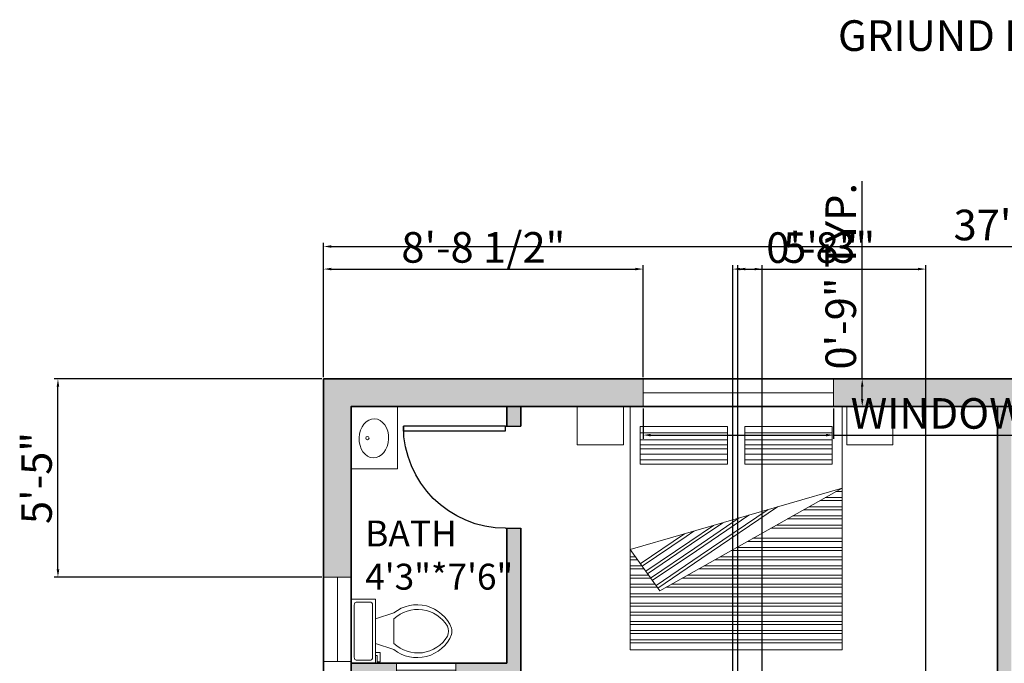
# Model space of a CAD drawing. Units: inches. Extents: x 1698 to 2352, y 1975 to 2732.
# Tile 3 of 4: x 1707 to 2029, y 2521 to 2732. Entities that reach past the tile are written whole.
import ezdxf

# ---------------------------------------------------------------- set-up
doc = ezdxf.new("R2010")
doc.units = ezdxf.units.IN
for name, color, linetype, lineweight in [('A-ANNO-DIMS', 2, 'Continuous', 18), ('A-ANNO-TEXT', 7, 'Continuous', 25), ('A-AREA-IDEN', 7, 'Continuous', 18), ('A-FLOR-FIXT', 231, 'Continuous', 18), ('A-WALL-PATT', 52, 'Continuous', 13), ('door', 80, 'Continuous', 25), ('fur', 10, 'Continuous', 18), ('wall', 7, 'Continuous', 35), ('window', 130, 'Continuous', 18)]:
    doc.layers.add(name, color=color, linetype=linetype, lineweight=lineweight)
doc.styles.get("Standard").update_dxf_attribs({"font": 'arial.ttf'})
doc.dimstyles.new('ISO-25', dxfattribs={"dimtxt": 10, "dimasz": 2.5, "dimexe": 1.25, "dimexo": 0.625, "dimtad": 1, "dimdec": 0, "dimlunit": 4, "dimtxsty": 'Standard', "dimcen": 2.5, "dimadec": 0, "dimazin": 0, "dimtfac": 1, "dimtdec": 0, "dimtmove": 0, "dimatfit": 3, "dimfxl": 1, "dimarcsym": 0})

# ---------------------------------------------------------------- blocks, each defined once
blk = doc.blocks.new('*U2')
for p, q in [((0, 0), (0, -6)), ((40, 0), (40, -6))]:
    blk.add_line(p, q)
blk.add_lwpolyline([(0, 0), (0, 40), (1.75, 40), (1.75, 0)], close=True)
blk.add_arc((0, 0), 40, 0, 90)
blk = doc.blocks.new('*U4')
for p, q in [((9.5, -6), (9.5, -2)), ((-10, -8.5), (-8, -8.5)), ((-10, -9.5), (-10, -8.5)), ((-7, -9.5), (-10, -9.5)), ((-8, -8.5), (-8, -8)), ((-7, -8), (-7, -9.5)), ((-4, -8), (-6, -14)), ((4, -8), (6, -14)), ((4, -14), (-4, -14))]:
    blk.add_line(p, q)
blk.add_lwpolyline([(10.5, -8), (10.5, 0), (-10.5, 0), (-10.5, -8)], close=True)
for points in [[(-9.5, -2), (-9.5, -6)], [(8.5, -1), (-8.5, -1)], [(-8.5, -7), (8.5, -7)]]:
    blk.add_lwpolyline(points)
for centre, radius, start, end in [((-8.62, -1.88), 0.884, 81.8699, 188.1301), ((8.62, -1.88), 0.884, 351.8699, 98.1301), ((-8.62, -6.12), 0.884, 171.8699, 278.1301), ((8.62, -6.12), 0.884, 261.8699, 8.1301), ((3.52, -21.58), 12.17, 141.4691, 247.9714), ((4.2, -21.82), 11.33, 136.3677, 238.9468), ((-3.52, -21.58), 12.17, 292.0284, 38.5307), ((-4.2, -21.82), 11.33, 301.053, 43.6321), ((0, -27.88), 4, 245.7318, 294.2682), ((0, -29), 4, 254.8605, 285.1395)]:
    blk.add_arc(centre, radius, start, end)
blk = doc.blocks.new('*D7')
at = {"layer": 'A-ANNO-DIMS', "color": 0, "lineweight": -2, "transparency": 16777216}
for p, q in [((1805.99, 2614.89), (1805.99, 2658.85)), ((2255.99, 2614.89), (2255.99, 2658.85)), ((1808.49, 2657.6), (2253.49, 2657.6))]:
    blk.add_line(p, q, dxfattribs=at)
at = {"layer": 'A-ANNO-DIMS', "color": 0, "lineweight": 100, "transparency": 16777216}
for points in [[(1808.49, 2658.02), (1808.49, 2657.18), (1805.99, 2657.6)], [(2253.49, 2658.02), (2253.49, 2657.18), (2255.99, 2657.6)]]:
    blk.add_solid(points, dxfattribs=at)
at = {"layer": 'Defpoints', "color": 0, "lineweight": 100, "transparency": 16777216}
for p in [(2255.99, 2657.6), (1805.99, 2614.26), (2255.99, 2614.26)]:
    blk.add_point(p, dxfattribs=at)
at = {"layer": 'A-ANNO-DIMS', "color": 0, "transparency": 16777216, "insert": (2030.99, 2663.33), "char_height": 10, "attachment_point": 5}
blk.add_mtext('37\'-6"', dxfattribs=at)
blk = doc.blocks.new('BED-DOUBLE-WITH-NIGHTSTANDS')
for p, q in [((20.55, 70.98), (49.18, 70.98)), ((54.81, 70.98), (83.45, 70.98)), ((20.61, 68.69), (49.25, 68.69)), ((54.87, 68.69), (83.51, 68.69)), ((20.55, 67.05), (49.18, 67.05)), ((20.55, 65.74), (49.18, 65.74)), ((54.81, 67.05), (83.45, 67.05)), ((54.81, 65.74), (83.45, 65.74)), ((20.55, 63.98), (49.18, 63.98)), ((20.55, 62.15), (49.18, 62.15)), ((54.81, 63.98), (83.45, 63.98)), ((54.81, 62.15), (83.45, 62.15)), ((17.28, 32.76), (86.63, 52.89)), ((86.63, 52.89), (27, 19.28)), ((84.66, 51.78), (86.63, 51.78)), ((86.25, 52.78), (86.63, 52.78)), ((79.34, 48.78), (86.63, 48.78)), ((81.11, 49.78), (86.63, 49.78)), ((40.19, 30.78), (62.43, 45.87)), ((40.75, 29.96), (65.55, 46.77)), ((74.02, 45.78), (86.63, 45.78)), ((75.79, 46.78), (86.63, 46.78)), ((38.42, 33.24), (53.01, 43.13)), ((38.98, 32.41), (56.13, 44.04)), ((68.7, 42.78), (86.63, 42.78)), ((70.47, 43.78), (86.63, 43.78)), ((35.61, 37.09), (38.16, 38.82)), ((36.83, 35.44), (44.53, 40.67)), ((37.39, 34.62), (47.65, 41.57)), ((63.38, 39.78), (86.63, 39.78)), ((65.15, 40.78), (86.63, 40.78)), ((20.62, 28.13), (35.05, 37.91)), ((21.18, 27.3), (35.61, 37.09)), ((55.69, 35.45), (86.63, 35.45)), ((57.46, 36.45), (86.63, 36.45)), ((27, 19.28), (17.28, 32.76)), ((17.28, 32.45), (17.5, 32.45)), ((22.4, 25.66), (36.83, 35.44)), ((22.96, 24.83), (37.39, 34.62)), ((23.99, 23.45), (38.42, 33.24)), ((24.55, 22.62), (38.98, 32.41)), ((50.37, 32.45), (86.63, 32.45)), ((52.14, 33.45), (86.63, 33.45)), ((17.28, 30.45), (18.94, 30.45)), ((17.28, 29.45), (19.66, 29.45)), ((25.76, 21), (40.19, 30.78)), ((26.32, 20.17), (40.75, 29.96)), ((45.05, 29.45), (86.63, 29.45)), ((46.82, 30.45), (86.63, 30.45)), ((17.28, 27.45), (21.11, 27.45)), ((17.28, 26.45), (21.83, 26.45)), ((39.73, 26.45), (86.63, 26.45)), ((41.5, 27.45), (86.63, 27.45)), ((17.28, 24.45), (23.27, 24.45)), ((17.28, 23.45), (23.99, 23.45)), ((34.41, 23.45), (86.63, 23.45)), ((36.18, 24.45), (86.63, 24.45)), ((17.28, 21.45), (25.43, 21.45)), ((17.28, 20.45), (26.16, 20.45)), ((29.09, 20.45), (86.63, 20.45)), ((30.86, 21.45), (86.63, 21.45)), ((17.28, 18.28), (86.63, 18.28)), ((17.28, 17.28), (86.63, 17.28)), ((17.28, 15.28), (86.63, 15.28)), ((17.28, 14.28), (86.63, 14.28)), ((17.28, 12.28), (86.63, 12.28)), ((17.28, 11.28), (86.63, 11.28)), ((17.28, 9.28), (86.63, 9.28)), ((17.28, 8.28), (86.63, 8.28)), ((17.28, 6.28), (86.63, 6.28)), ((17.28, 5.28), (86.63, 5.28)), ((17.28, 3.28), (86.63, 3.28)), ((17.28, 2.28), (86.63, 2.28))]:
    blk.add_line(p, q)
for points in [[(0, 79.57), (15.07, 79.57), (15.07, 67), (0, 67)], [(17.28, 79.57), (86.63, 79.57), (86.63, 0), (17.28, 0)], [(88.18, 79.57), (103.25, 79.57), (103.25, 67), (88.18, 67)], [(20.55, 73), (49.18, 73), (49.18, 60.76), (20.55, 60.76)], [(54.81, 73), (83.45, 73), (83.45, 60.76), (54.81, 60.76)]]:
    blk.add_lwpolyline(points, close=True)
blk = doc.blocks.new('BASIN-VANITY')
blk.add_lwpolyline([(0, 20.39), (15.22, 20.39), (15.22, 0), (0, 0)], close=True)
blk.add_circle((5.32, 10.07), 0.551)
blk.add_ellipse((7.43, 9.98), major_axis=(-0.23, -6.4), ratio=0.75221)
blk = doc.blocks.new('WIN-BATH-19_41')
blk.add_line((0, 2.25), (19.41, 2.25))
blk.add_lwpolyline([(0, 4.5), (19.41, 4.5), (19.41, 0), (0, 0)], close=True)
blk = doc.blocks.new('WIN-BATH-27_578')
blk.add_line((4.5, 0), (4.5, 27.58))
blk.add_lwpolyline([(0, 0), (9, 0), (9, 27.58), (0, 27.58)], close=True)
blk = doc.blocks.new('WIN-BEDROOM-62_374')
blk.add_line((0, 4.5), (62.37, 4.5))
blk.add_lwpolyline([(0, 0), (62.37, 0), (62.37, 9), (0, 9)], close=True)
blk = doc.blocks.new('*D20')
at = {"layer": 'A-ANNO-DIMS', "color": 0, "lineweight": -2, "transparency": 16777216}
for p, q in [((2046.1, 2605.26), (2046.1, 2693.32)), ((2060.97, 2605.26), (2044.85, 2605.26)), ((2046.1, 2528.19), (2046.1, 2602.76)), ((2060.97, 2525.69), (2044.85, 2525.69))]:
    blk.add_line(p, q, dxfattribs=at)
at = {"layer": 'A-ANNO-DIMS', "color": 0, "lineweight": 100, "transparency": 16777216}
for points in [[(2045.69, 2602.76), (2046.52, 2602.76), (2046.1, 2605.26)], [(2045.69, 2528.19), (2046.52, 2528.19), (2046.1, 2525.69)]]:
    blk.add_solid(points, dxfattribs=at)
at = {"layer": 'Defpoints', "color": 0, "lineweight": 100, "transparency": 16777216}
for p in [(2046.1, 2605.26), (2061.59, 2605.26), (2061.59, 2525.69)]:
    blk.add_point(p, dxfattribs=at)
at = {"layer": 'A-ANNO-DIMS', "color": 0, "transparency": 16777216, "insert": (2040.31, 2650.54), "char_height": 10, "attachment_point": 5, "rotation": 90}
blk.add_mtext('6\'-7 1/2" TYP.', dxfattribs=at)
blk = doc.blocks.new('*D29')
at = {"layer": 'A-ANNO-DIMS', "color": 0, "lineweight": -2, "transparency": 16777216}
for p, q in [((1910.52, 2604.64), (1910.52, 2594.66)), ((1972.89, 2604.64), (1972.89, 2594.66)), ((1913.02, 2595.91), (1970.39, 2595.91)), ((1972.89, 2595.91), (2126.48, 2595.91))]:
    blk.add_line(p, q, dxfattribs=at)
at = {"layer": 'A-ANNO-DIMS', "color": 0, "lineweight": 100, "transparency": 16777216}
for points in [[(1913.02, 2596.32), (1913.02, 2595.49), (1910.52, 2595.91)], [(1970.39, 2596.32), (1970.39, 2595.49), (1972.89, 2595.91)]]:
    blk.add_solid(points, dxfattribs=at)
at = {"layer": 'Defpoints', "color": 0, "lineweight": 100, "transparency": 16777216}
for p in [(1910.52, 2605.26), (1972.89, 2605.26), (1972.89, 2595.91)]:
    blk.add_point(p, dxfattribs=at)
at = {"layer": 'A-ANNO-DIMS', "color": 0, "transparency": 16777216, "insert": (2050.94, 2601.7), "char_height": 10, "attachment_point": 5}
blk.add_mtext('WINDOW 5\'-2 1/2" TYP.', dxfattribs=at)
blk = doc.blocks.new('*D30')
at = {"layer": 'A-ANNO-DIMS', "color": 0, "lineweight": -2, "transparency": 16777216}
for p, q in [((1982.25, 2614.26), (1982.25, 2678.97)), ((1973.52, 2614.26), (1983.5, 2614.26)), ((1982.25, 2607.76), (1982.25, 2611.76)), ((1973.52, 2605.26), (1983.5, 2605.26))]:
    blk.add_line(p, q, dxfattribs=at)
at = {"layer": 'A-ANNO-DIMS', "color": 0, "lineweight": 100, "transparency": 16777216}
for points in [[(1981.83, 2611.76), (1982.66, 2611.76), (1982.25, 2614.26)], [(1981.83, 2607.76), (1982.66, 2607.76), (1982.25, 2605.26)]]:
    blk.add_solid(points, dxfattribs=at)
at = {"layer": 'Defpoints', "color": 0, "lineweight": 100, "transparency": 16777216}
for p in [(1972.89, 2614.26), (1982.25, 2614.26), (1972.89, 2605.26)]:
    blk.add_point(p, dxfattribs=at)
at = {"layer": 'A-ANNO-DIMS', "color": 0, "transparency": 16777216, "insert": (1976.52, 2647.86), "char_height": 10, "attachment_point": 5, "rotation": 90}
blk.add_mtext('0\'-9" TYP.', dxfattribs=at)
blk = doc.blocks.new('*D36')
at = {"layer": 'A-ANNO-DIMS', "color": 0, "lineweight": -2, "transparency": 16777216}
for p, q in [((1941.49, 2286.14), (1941.49, 2651.46)), ((1943.99, 2650.21), (1946.99, 2650.21)), ((1949.49, 2286.14), (1949.49, 2651.46)), ((1949.49, 2650.21), (1979.82, 2650.21))]:
    blk.add_line(p, q, dxfattribs=at)
at = {"layer": 'A-ANNO-DIMS', "color": 0, "lineweight": 100, "transparency": 16777216}
for points in [[(1943.99, 2650.63), (1943.99, 2649.8), (1941.49, 2650.21)], [(1946.99, 2650.63), (1946.99, 2649.8), (1949.49, 2650.21)]]:
    blk.add_solid(points, dxfattribs=at)
at = {"layer": 'Defpoints', "color": 0, "lineweight": 100, "transparency": 16777216}
for p in [(1949.49, 2650.21), (1941.49, 2285.51), (1949.49, 2285.51)]:
    blk.add_point(p, dxfattribs=at)
at = {"layer": 'A-ANNO-DIMS', "color": 0, "transparency": 16777216, "insert": (1965.91, 2655.94), "char_height": 10, "attachment_point": 5}
blk.add_mtext('0\'-8"', dxfattribs=at)
blk = doc.blocks.new('*D40')
at = {"layer": 'A-ANNO-DIMS', "color": 0, "lineweight": -2, "transparency": 16777216}
for p, q in [((1805.99, 2614.89), (1805.99, 2651.46)), ((1808.49, 2650.21), (1908.02, 2650.21)), ((1910.52, 2614.89), (1910.52, 2651.46))]:
    blk.add_line(p, q, dxfattribs=at)
at = {"layer": 'A-ANNO-DIMS', "color": 0, "lineweight": 100, "transparency": 16777216}
for points in [[(1808.49, 2650.63), (1808.49, 2649.8), (1805.99, 2650.21)], [(1908.02, 2650.63), (1908.02, 2649.8), (1910.52, 2650.21)]]:
    blk.add_solid(points, dxfattribs=at)
at = {"layer": 'Defpoints', "color": 0, "lineweight": 100, "transparency": 16777216}
for p in [(1910.52, 2650.21), (1805.99, 2614.26), (1910.52, 2614.26)]:
    blk.add_point(p, dxfattribs=at)
at = {"layer": 'A-ANNO-DIMS', "color": 0, "transparency": 16777216, "insert": (1858.25, 2656.01), "char_height": 10, "attachment_point": 5}
blk.add_mtext('8\'-8 1/2"', dxfattribs=at)
blk = doc.blocks.new('*D43')
at = {"layer": 'A-ANNO-DIMS', "color": 0, "lineweight": -2, "transparency": 16777216}
for p, q in [((1805.37, 2614.26), (1717.79, 2614.26)), ((1719.04, 2551.97), (1719.04, 2611.76)), ((1805.37, 2549.47), (1717.79, 2549.47))]:
    blk.add_line(p, q, dxfattribs=at)
at = {"layer": 'A-ANNO-DIMS', "color": 0, "lineweight": 100, "transparency": 16777216}
for points in [[(1718.62, 2611.76), (1719.46, 2611.76), (1719.04, 2614.26)], [(1718.62, 2551.97), (1719.46, 2551.97), (1719.04, 2549.47)]]:
    blk.add_solid(points, dxfattribs=at)
at = {"layer": 'Defpoints', "color": 0, "lineweight": 100, "transparency": 16777216}
for p in [(1719.04, 2614.26), (1805.99, 2614.26), (1805.99, 2549.47)]:
    blk.add_point(p, dxfattribs=at)
at = {"layer": 'A-ANNO-DIMS', "color": 0, "transparency": 16777216, "insert": (1713.33, 2581.87), "char_height": 10, "attachment_point": 5, "rotation": 90}
blk.add_mtext('5\'-5"', dxfattribs=at)
blk = doc.blocks.new('*D50')
at = {"layer": 'A-ANNO-DIMS', "color": 0, "lineweight": -2, "transparency": 16777216}
for p, q in [((1939.87, 2337.39), (1939.87, 2651.46)), ((1942.37, 2650.21), (2000.54, 2650.21)), ((2003.04, 2337.39), (2003.04, 2651.46))]:
    blk.add_line(p, q, dxfattribs=at)
at = {"layer": 'A-ANNO-DIMS', "color": 0, "lineweight": 100, "transparency": 16777216}
for points in [[(1942.37, 2650.63), (1942.37, 2649.8), (1939.87, 2650.21)], [(2000.54, 2650.63), (2000.54, 2649.8), (2003.04, 2650.21)]]:
    blk.add_solid(points, dxfattribs=at)
at = {"layer": 'Defpoints', "color": 0, "lineweight": 100, "transparency": 16777216}
for p in [(2003.04, 2650.21), (1939.87, 2336.76), (2003.04, 2336.76)]:
    blk.add_point(p, dxfattribs=at)
at = {"layer": 'A-ANNO-DIMS', "color": 0, "transparency": 16777216, "insert": (1971.45, 2655.95), "char_height": 10, "attachment_point": 5}
blk.add_mtext('5\'-3"', dxfattribs=at)

msp = doc.modelspace()

# ---------------------------------------------------------------- hatches: boundary and pattern name
at = {"layer": 'A-WALL-PATT'}
h = msp.add_hatch(color=256, dxfattribs=at)
h.dxf.hatch_style = 1
h.paths.add_polyline_path([(1910.52, 2614.26), (1805.99, 2614.26), (1805.99, 2549.47), (1814.99, 2549.47), (1814.99, 2605.26), (1910.52, 2605.26)])
h.paths.add_polyline_path([(2084.19, 2614.26), (1972.89, 2614.26), (1972.89, 2605.26), (2026.49, 2605.26), (2084.19, 2605.26)])
h.paths.add_polyline_path([(2255.99, 2614.26), (2146.56, 2614.26), (2146.56, 2605.26), (2148.21, 2605.26), (2186.99, 2605.26), (2246.99, 2605.26), (2246.99, 2546.53), (2255.99, 2546.53)])
h.paths.add_polyline_path([(2191.49, 2605.26), (2186.99, 2605.26), (2186.99, 2595.02), (2191.49, 2595.02)], flags=17)
h.paths.add_polyline_path([(2191.49, 2563.28), (2186.99, 2563.28), (2186.99, 2510.76), (2191.49, 2510.76)])
h.paths.add_polyline_path([(2246.99, 2515.26), (2191.49, 2515.26), (2191.49, 2510.76), (2246.99, 2510.76)])
h.paths.add_polyline_path([(2030.99, 2605.26), (2026.49, 2605.26), (2026.49, 2473.26), (2020.85, 2473.26), (2020.85, 2468.76), (2030.99, 2468.76)])
h.paths.add_polyline_path([(1980.85, 2473.26), (1870.49, 2473.26), (1865.99, 2473.26), (1865.99, 2468.76), (1980.85, 2468.76)])
h.paths.add_polyline_path([(1828.36, 2413.26), (1814.99, 2413.26), (1814.99, 2408.76), (1828.36, 2408.76)])
h.paths.add_polyline_path([(1865.99, 2413.26), (1847.77, 2413.26), (1847.77, 2408.76), (1865.99, 2408.76)])
h.paths.add_polyline_path([(1870.49, 2418.36), (1865.99, 2418.36), (1865.99, 2372.57), (1870.49, 2372.57)])
h.paths.add_polyline_path([(2036.32, 2473.26), (2030.99, 2473.26), (2030.99, 2468.76), (2036.32, 2468.76)])
h.paths.add_polyline_path([(2191.49, 2473.26), (2186.99, 2473.26), (2076.32, 2473.26), (2076.32, 2468.76), (2191.49, 2468.76)])
h.paths.add_polyline_path([(2246.99, 2471.76), (2191.49, 2471.76), (2191.49, 2468.76), (2246.99, 2468.76)])
h.paths.add_polyline_path([(2255.99, 2406.37), (2246.99, 2406.37), (2246.99, 2404.25), (2246.99, 2336.76), (2246.99, 2083.26), (2127.92, 2083.26), (2127.92, 2074.26), (2255.99, 2074.26)])
h.paths.add_polyline_path([(2110.49, 2336.76), (2083.04, 2336.76), (2083.04, 2336.67), (2083.04, 2332.26), (2110.49, 2332.26)])
h.paths.add_polyline_path([(2024.3, 2336.76), (2003.04, 2336.76), (2003.04, 2332.26), (2024.3, 2332.26)])
h.paths.add_polyline_path([(2246.99, 2164.26), (2216.76, 2164.26), (2216.76, 2155.26), (2246.99, 2155.26)], flags=17)
h.paths.add_polyline_path([(1958.99, 2083.26), (1927.89, 2083.26), (1927.89, 2074.26), (1958.99, 2074.26)])
h.paths.add_polyline_path([(1963.49, 2185.34), (1958.99, 2185.34), (1958.99, 2083.26), (1963.49, 2083.26)])
h.paths.add_polyline_path([(1963.49, 2238.76), (1855.03, 2238.76, -0.010403), (1855.05, 2237.79), (1855.05, 2234.26), (1958.99, 2234.26), (1958.99, 2225.34), (1963.49, 2225.34)])
h.paths.add_polyline_path([(1831.56, 2237.79), (1831.56, 2238.76), (1814.99, 2238.76), (1814.99, 2234.26), (1831.56, 2234.26)])
h.paths.add_polyline_path([(1939.87, 2336.76), (1814.99, 2336.76), (1814.99, 2332.26), (1856.99, 2332.26), (1939.87, 2332.26)])
h.paths.add_polyline_path([(1814.99, 2377.93), (1805.99, 2377.93), (1805.99, 2325.81), (1814.99, 2325.81)])
h.paths.add_polyline_path([(1829.84, 2521.26), (1814.99, 2521.26), (1814.99, 2516.76), (1829.84, 2516.76)])
h.paths.add_polyline_path([(2255.99, 2471.76), (2246.99, 2471.76), (2246.99, 2438.09), (2255.99, 2438.09)])
h = msp.add_hatch(color=256, dxfattribs=at)
h.dxf.hatch_style = 1
h.paths.add_polyline_path([(1870.49, 2565.42), (1865.99, 2565.42), (1865.99, 2521.26), (1849.25, 2521.26), (1849.25, 2516.76), (1870.49, 2516.76)])
h.paths.add_polyline_path([(1870.49, 2605.26), (1865.99, 2605.26), (1865.99, 2598.8), (1870.49, 2598.8)])
h.paths.add_polyline_path([(2246.99, 2336.76), (2147.99, 2336.76), (2147.99, 2360.76), (2147.99, 2418.65), (2143.49, 2418.65), (2143.49, 2332.26), (2246.99, 2332.26)])
h.paths.add_polyline_path([(2143.49, 2336.76), (2110.49, 2336.76), (2110.49, 2325.07), (2114.99, 2325.07), (2114.99, 2332.26), (2143.49, 2332.26)])
h.paths.add_polyline_path([(2114.99, 2285.07), (2110.49, 2285.07), (2110.49, 2155.26), (2141.76, 2155.26), (2141.76, 2164.26), (2114.99, 2164.26)])
h.paths.add_polyline_path([(1814.99, 2298.28), (1805.99, 2298.28), (1805.99, 2074.26), (1852.89, 2074.26), (1852.89, 2083.26), (1814.99, 2083.26)])

# ---------------------------------------------------------------- linework, layer by layer
at = {"layer": 'wall'}
for p, q in [((1814.99, 2605.26), (1814.99, 2521.26)), ((1865.99, 2598.8), (1865.99, 2605.26)), ((1870.49, 2605.26), (2026.49, 2605.26)), ((1870.49, 2598.8), (1870.49, 2605.26)), ((2026.49, 2605.26), (2026.49, 2473.26)), ((1865.99, 2521.26), (1865.99, 2565.42)), ((1870.49, 2516.76), (1870.49, 2565.42)), ((1814.99, 2521.26), (1865.99, 2521.26))]:
    msp.add_line(p, q, dxfattribs=at)
for points in [[(2127.92, 2074.26), (2255.99, 2074.26), (2255.99, 2614.26), (1805.99, 2614.26), (1805.99, 2074.26), (1958.99, 2074.26)], [(2127.92, 2083.26), (2246.99, 2083.26), (2246.99, 2605.26), (1814.99, 2605.26), (1814.99, 2516.76)]]:
    msp.add_lwpolyline(points, dxfattribs=at)

# ---------------------------------------------------------------- block references
at = {"layer": 'A-FLOR-FIXT'}
msp.add_blockref('BASIN-VANITY', (1814.99, 2584.87), dxfattribs=at)
at = {"layer": 'A-FLOR-FIXT', "rotation": 90}
msp.add_blockref('*U4', (1814.99, 2531.76), dxfattribs=at)
at = {"layer": 'door', "xscale": -0.8344442270959994, "yscale": 0.8344442270959994, "zscale": 0.8344442270959994, "rotation": 90}
msp.add_blockref('*U2', (1865.48, 2598.8), dxfattribs=at)
at = {"layer": 'fur'}
msp.add_blockref('BED-DOUBLE-WITH-NIGHTSTANDS', (1889, 2525.69), dxfattribs=at)
at = {"layer": 'window'}
for name, p in [('WIN-BEDROOM-62_374', (1910.52, 2605.26)), ('WIN-BATH-27_578', (1805.99, 2521.89)), ('WIN-BATH-19_41', (1829.84, 2516.76))]:
    msp.add_blockref(name, p, dxfattribs=at)

# ---------------------------------------------------------------- texts
at = {"layer": 'A-ANNO-TEXT', "insert": (1974.3, 2731.6), "char_height": 10.0406, "attachment_point": 1}
msp.add_mtext_dynamic_manual_height_columns('GRIUND FLOOR PLAN', width=1490.6775, gutter_width=50.2, heights=[0], dxfattribs=at)
at = {"layer": 'A-AREA-IDEN', "insert": (1819.58, 2567.96), "char_height": 8.476, "attachment_point": 1}
msp.add_mtext_dynamic_manual_height_columns('BATH\\P4\'3"*7\'6"', width=272.6258, gutter_width=42.38, heights=[0], dxfattribs=at)

# ---------------------------------------------------------------- dimensions: what is measured, and where the dimension line sits
at = {"layer": 'A-ANNO-DIMS'}
for base, p1, p2, picture, middle in [((2046.1, 2605.26), (2061.59, 2525.69), (2061.59, 2605.26), '*D20', (2040.31, 2650.54)), ((1982.25, 2614.26), (1972.89, 2605.26), (1972.89, 2614.26), '*D30', (1976.52, 2647.86))]:
    dim = msp.add_linear_dim(base=base, p1=p1, p2=p2, angle=90, text='<> TYP.', dimstyle='ISO-25', override={"dimdec": 1, "dimlfac": 1, "dimrnd": 0, "dimzin": 1, "dimdsep": 46, "dimlunit": 4, "dimfrac": 2}, dxfattribs=at)
    dim.commit()
    dim.dimension.update_dxf_attribs({"geometry": picture, "text_midpoint": middle})
for base, p1, p2, override, picture, middle in [((1910.52, 2650.21), (1805.99, 2614.26), (1910.52, 2614.26), {"dimdec": 1, "dimlfac": 1, "dimrnd": 0, "dimzin": 1, "dimdsep": 46, "dimlunit": 4, "dimfrac": 2}, '*D40', (1858.25, 2656.01)), ((2255.99, 2657.6), (1805.99, 2614.26), (2255.99, 2614.26), {"dimclrd": 0, "dimclre": 0, "dimclrt": 0}, '*D7', (2030.99, 2663.33)), ((2003.04, 2650.21), (1939.87, 2336.76), (2003.04, 2336.76), {"dimdec": 1, "dimlfac": 1, "dimrnd": 0, "dimzin": 1, "dimdsep": 46, "dimlunit": 4, "dimfrac": 2}, '*D50', (1971.45, 2655.95)), ((1949.49, 2650.21), (1941.49, 2285.51), (1949.49, 2285.51), {"dimdec": 1, "dimlfac": 1, "dimrnd": 0, "dimzin": 1, "dimdsep": 46, "dimlunit": 4, "dimfrac": 2}, '*D36', (1965.91, 2655.94))]:
    dim = msp.add_linear_dim(base=base, p1=p1, p2=p2, dimstyle='ISO-25', override=override, dxfattribs=at)
    dim.commit()
    dim.dimension.update_dxf_attribs({"geometry": picture, "text_midpoint": middle})
dim = msp.add_linear_dim(base=(1972.89, 2595.91), p1=(1910.52, 2605.26), p2=(1972.89, 2605.26), text='WINDOW <> TYP.', dimstyle='ISO-25', override={"dimdec": 1, "dimlfac": 1, "dimrnd": 0, "dimzin": 1, "dimdsep": 46, "dimlunit": 4, "dimfrac": 2}, dxfattribs=at)
dim.commit()
dim.dimension.update_dxf_attribs({"geometry": '*D29', "text_midpoint": (2050.94, 2601.7)})
dim = msp.add_linear_dim(base=(1719.04, 2614.26), p1=(1805.99, 2549.47), p2=(1805.99, 2614.26), angle=90, dimstyle='ISO-25', override={"dimdec": 1, "dimlfac": 1, "dimrnd": 0, "dimzin": 1, "dimdsep": 46, "dimlunit": 4, "dimfrac": 2}, dxfattribs=at)
dim.commit()
dim.dimension.update_dxf_attribs({"geometry": '*D43', "text_midpoint": (1713.33, 2581.87)})

doc.saveas('drawing.dxf')
